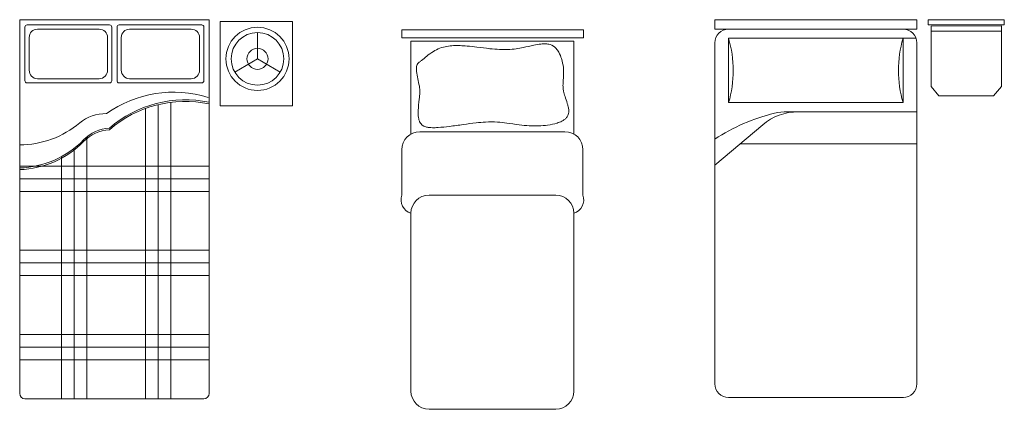
# Model space of a CAD drawing. Units: inches. Extents: x 1994 to 3075, y 3517 to 3950.
# Tile 11 of 58: x 1994.3296 to 1994.5407, y 3553.2315 to 3553.315. Entities that reach past the tile are written whole.
import ezdxf

# ---------------------------------------------------------------- set-up
doc = ezdxf.new("R2010")
doc.units = ezdxf.units.IN
doc.layers.add('A-FURN-REFR', color=8, linetype='Continuous', lineweight=13)

msp = doc.modelspace()

# ---------------------------------------------------------------- linework, layer by layer
at = {"layer": 'A-FURN-REFR'}
for p, q in [((1994.370185678926, 3553.314964244441), (1994.329576990967, 3553.314964244441)), ((1994.329576990967, 3553.314964244441), (1994.329576990967, 3553.234874887633)), ((1994.348866117747, 3553.313836225331), (1994.331156217721, 3553.313836225331)), ((1994.368606452172, 3553.313836225331), (1994.350896552145, 3553.313836225331)), ((1994.370185678926, 3553.314964244441), (1994.370185678926, 3553.234874887633)), ((1994.478602848426, 3553.314914551347), (1994.521910079674, 3553.314920144558)), ((1994.478603102663, 3553.312946047427), (1994.478602848426, 3553.314914551347)), ((1994.521910188973, 3553.312950623674), (1994.521910079674, 3553.314920144558)), ((1994.52435569552, 3553.314916554879), (1994.540668217137, 3553.314918661672)), ((1994.524355834575, 3553.313839871399), (1994.52435569552, 3553.314916554879)), ((1994.524355834575, 3553.313839871399), (1994.540668356192, 3553.313841978191)), ((1994.5249825969, 3553.313615310058), (1994.540041651892, 3553.313617254961)), ((1994.540041651892, 3553.313617254961), (1994.54004332985, 3553.300625129086)), ((1994.540668356192, 3553.313841978191), (1994.540668217137, 3553.314918661671)), ((1994.330705010077, 3553.313385017688), (1994.330705010077, 3553.301879222766)), ((1994.346610079528, 3553.312933810043), (1994.333412255941, 3553.312933810043)), ((1994.349317325391, 3553.301879222766), (1994.349317325391, 3553.313385017688)), ((1994.350445344501, 3553.313385017688), (1994.350445344501, 3553.301879222766)), ((1994.366350413952, 3553.312933810043), (1994.353152590365, 3553.312933810043)), ((1994.369057659816, 3553.301879222766), (1994.369057659816, 3553.313385017688)), ((1994.38056212126, 3553.312215362403), (1994.38056212126, 3553.306575266854)), ((1994.478603102663, 3553.312946047427), (1994.521910188842, 3553.312951640618)), ((1994.5249825969, 3553.313615310058), (1994.524984274856, 3553.300623184182)), ((1994.524982738188, 3553.312521342884), (1994.540041793181, 3553.312523287789)), ((1994.331607425365, 3553.311128979467), (1994.331607425365, 3553.304135260986)), ((1994.348414910103, 3553.304135260986), (1994.348414910103, 3553.311128979467)), ((1994.351347759789, 3553.311128979467), (1994.351347759789, 3553.304135260986)), ((1994.368155244528, 3553.304135260986), (1994.368155244528, 3553.311128979467)), ((1994.448401600234, 3553.310391664947), (1994.413453017272, 3553.310391664947)), ((1994.413453017272, 3553.310391664947), (1994.413453017272, 3553.290455538603)), ((1994.448401600234, 3553.310391664947), (1994.448401600234, 3553.290455538603)), ((1994.478612611088, 3553.236961796068), (1994.478603484016, 3553.309993291545)), ((1994.521741212387, 3553.31098311484), (1994.481556112778, 3553.310977924859)), ((1994.481556112778, 3553.310977924859), (1994.48155789243, 3553.297198397415)), ((1994.518959466981, 3553.297202210954), (1994.518957687329, 3553.310981738399)), ((1994.521910570327, 3553.309997867792), (1994.521919697399, 3553.236966372316)), ((1994.375677655234, 3553.303755219079), (1994.38056212126, 3553.306575266854)), ((1994.385446587286, 3553.303755219079), (1994.38056212126, 3553.306575266854)), ((1994.331156217721, 3553.301428015121), (1994.348866117747, 3553.301428015121)), ((1994.333412255941, 3553.30233043041), (1994.346610079528, 3553.30233043041)), ((1994.350896552145, 3553.301428015121), (1994.368606452172, 3553.301428015121)), ((1994.353152590365, 3553.30233043041), (1994.366350413952, 3553.30233043041)), ((1994.524984274856, 3553.300623184182), (1994.526657757425, 3553.298654896362)), ((1994.538370355752, 3553.298656409065), (1994.54004332985, 3553.300625129086)), ((1994.359289826759, 3553.296769779996), (1994.359289826759, 3553.233746868524)), ((1994.361997072623, 3553.297259562664), (1994.361997072623, 3553.233746868524)), ((1994.48155789243, 3553.297198397415), (1994.518959170259, 3553.29720322786)), ((1994.526657757425, 3553.298654896362), (1994.538370355752, 3553.298656409065)), ((1994.356582580895, 3553.295958376947), (1994.356582580895, 3553.233746868524)), ((1994.521912476966, 3553.295235105331), (1994.49414155207, 3553.295231518664)), ((1994.446460012292, 3553.290975785524), (1994.415394605214, 3553.290975785524)), ((1994.478606866596, 3553.283802582117), (1994.488875350771, 3553.292453532399)), ((1994.343948766863, 3553.289817339641), (1994.343948766863, 3553.233746868524)), ((1994.521913366791, 3553.288345341608), (1994.484019666392, 3553.288340447566)), ((1994.341241520999, 3553.28740160715), (1994.341241520999, 3553.233746868524)), ((1994.411511429329, 3553.28709260964), (1994.411511429329, 3553.277384669928)), ((1994.450343188176, 3553.277384669928), (1994.450343188176, 3553.28709260964)), ((1994.338534275135, 3553.285640265894), (1994.338534275135, 3553.233746868524)), ((1994.370185678926, 3553.283605313184), (1994.329576990967, 3553.283605313184)), ((1994.370185678926, 3553.28089806732), (1994.329576990967, 3553.28089806732)), ((1994.370185678926, 3553.278190821456), (1994.329576990967, 3553.278190821456)), ((1994.417336193156, 3553.277384669928), (1994.444518424349, 3553.277384669928)), ((1994.413453017272, 3553.273501494043), (1994.413453017272, 3553.235376388787)), ((1994.448401600234, 3553.235376388787), (1994.448401600234, 3553.273501494043)), ((1994.370185678926, 3553.265557007425), (1994.329576990967, 3553.265557007425)), ((1994.370185678926, 3553.262849761561), (1994.329576990967, 3553.262849761561)), ((1994.370185678926, 3553.260142515696), (1994.329576990967, 3553.260142515696)), ((1994.370185678926, 3553.247508701665), (1994.329576990967, 3553.247508701665)), ((1994.370185678926, 3553.244801455801), (1994.329576990967, 3553.244801455801)), ((1994.370185678926, 3553.242094209937), (1994.329576990967, 3553.242094209937)), ((1994.369057659816, 3553.233746868524), (1994.330705010077, 3553.233746868524)), ((1994.519044811687, 3553.234014262032), (1994.481565748322, 3553.23400942154)), ((1994.417336193156, 3553.231493212902), (1994.444518424349, 3553.231493212902))]:
    msp.add_line(p, q, dxfattribs=at)
for points in [[(1994.388077714789, 3553.314567166401), (1994.372579103558, 3553.314567166401), (1994.372579103558, 3553.296485896745), (1994.388077714789, 3553.296485896745)], [(1994.411513799174, 3553.311101471077), (1994.450430347792, 3553.311101471077), (1994.450430347792, 3553.312763276653), (1994.411513799174, 3553.312763276653)]]:
    msp.add_lwpolyline(points, close=True, dxfattribs=at)
msp.add_lwpolyline([(1994.415717140901, 3553.306221031559, -0.0071144536033679), (1994.416830524292, 3553.307136923001, -0.0291750801621191), (1994.418272017925, 3553.308160858666, -0.0995108413985327), (1994.421172431712, 3553.30925043835, -0.0309960537166681), (1994.422580733602, 3553.309406082746, -0.0213742242213407), (1994.424025083548, 3553.309416868291, -0.0138154102423473), (1994.425477869293, 3553.30932585958, -0.0092840040629771), (1994.427616086483, 3553.30909097738, 0.0043536539427215), (1994.430382063773, 3553.308755920688, 0.014634740864433), (1994.43244936847, 3553.308592984115, 0.0438384142680896), (1994.436015633939, 3553.308726752635, 0.0205965805776953), (1994.437522836489, 3553.308989654272, -0.0030532405795762), (1994.43982883519, 3553.309510514755, -0.0258862363996294), (1994.441307999698, 3553.30975390412, -0.0372674858245903), (1994.442342421448, 3553.309787357306, -0.0594222537962098), (1994.443283315345, 3553.309630668138, -0.1390712479793723), (1994.444575160915, 3553.308807129298, -0.0586638411555205), (1994.445166100647, 3553.307983348355, -0.0528613955005662), (1994.445743360173, 3553.306621725756, -0.0903311740027589), (1994.446177062131, 3553.302810669614, 0.0023761187996274), (1994.446069543849, 3553.301409835136, 0.0350786422935007), (1994.446080262775, 3553.300361830441, 0.0301021961769406), (1994.446193545359, 3553.299637858405, 0.0242628626286148), (1994.446496227885, 3553.298521961266, -0.0025129695723871), (1994.446969847513, 3553.297043305117, -0.016683843633439), (1994.447160354396, 3553.296335872206, -0.031042526979895), (1994.447274765204, 3553.295666265365, -0.1077433275196103), (1994.447189851161, 3553.294622835333, -0.0971969509952781), (1994.446835994608, 3553.294004616111, -0.0572188880031632), (1994.446385582422, 3553.293587640181, -0.0413009457476749), (1994.445812123817, 3553.293234952154, -0.0430763729579249), (1994.444773120372, 3553.292816983652, -0.0420582544055731), (1994.442762307514, 3553.292380438816, -0.0495548008396401), (1994.438805955694, 3553.292239582801, -0.0176483592672042), (1994.436665275761, 3553.292444104455, -0.0018432574081804), (1994.433985367609, 3553.292815578701, 0.0158524255451982), (1994.43204139292, 3553.293019261201, 0.0296706768072246), (1994.429448007234, 3553.293025570407, 0.0142130398266808), (1994.427456086711, 3553.29286037947, 0.0071404775766546), (1994.424675961824, 3553.292507505704, -0.0039170474728025), (1994.421683320919, 3553.292110452283, -0.0124176775830428), (1994.419263257741, 3553.291861204865, -0.0214267812853995), (1994.41806435162, 3553.291824593835, -0.0259849889690267), (1994.417321753347, 3553.291875388679, -0.0396653445020058), (1994.416653118596, 3553.292009335013, -0.2391240642373063), (1994.415323131073, 3553.293094547253, -0.0526178150763782), (1994.415128082925, 3553.293693775242, -0.0348338633937756), (1994.415030081924, 3553.294379871292, -0.0316331286276026), (1994.415020000411, 3553.2955210265, -0.0170430167712775), (1994.415237932306, 3553.297918818028, 0.0194593935250652), (1994.415342939074, 3553.2993814271, 0.0425716315945425), (1994.415270391061, 3553.30073702966, -0.0315728479582929), (1994.41467866575, 3553.303884359247, -0.0408804555025011), (1994.414648081667, 3553.304650098184, -0.0594404672514954), (1994.414737112971, 3553.305180186531, -0.1725909739171879), (1994.415225176221, 3553.305856330223, 0.01273912279684), (1994.415717140901, 3553.306221031559)], format="xyb", dxfattribs=at)
for radius in [0.0067681146598248, 0.005640095549854, 0.0022560382199416]:
    msp.add_circle((1994.38056212126, 3553.306575266854), radius, dxfattribs=at)
for centre, radius, start, end in [((1994.331156217721, 3553.313385017688), 0.0004512076439886, 90, 180), ((1994.348866117747, 3553.313385017688), 0.0004512076439886, 0, 90), ((1994.350896552145, 3553.313385017688), 0.0004512076439886, 90, 180), ((1994.368606452172, 3553.313385017688), 0.0004512076439886, 0, 90), ((1994.333412255941, 3553.311128979467), 0.0018048305759536, 90, 180), ((1994.346610079528, 3553.311128979467), 0.0018048305759529, 0, 90), ((1994.353152590365, 3553.311128979467), 0.0018048305759536, 90, 180), ((1994.366350413952, 3553.311128979467), 0.0018048305759529, 0, 90), ((1994.333412255941, 3553.304135260986), 0.0018048305759529, 180, 270), ((1994.346610079528, 3553.304135260986), 0.0018048305759529, 270, 0), ((1994.353152590365, 3553.304135260986), 0.0018048305759529, 180, 270), ((1994.366350413952, 3553.304135260986), 0.0018048305759529, 270, 0), ((1994.331156217721, 3553.301879222766), 0.0004512076439886, 180, 270), ((1994.348866117747, 3553.301879222766), 0.0004512076439879, 270, 0), ((1994.350896552145, 3553.301879222766), 0.0004512076439886, 180, 270), ((1994.368606452172, 3553.301879222766), 0.0004512076439879, 270, 0), ((1994.362573607713, 3553.274580434349), 0.0248643078922148, 72.67323284139673, 125.4131583510985), ((1994.365063151315, 3553.272935583567), 0.0248643078922151, 78.11082488000187, 130.8507503895504), ((1994.365063151315, 3553.272585021769), 0.0248643078922151, 78.11082488000187, 130.8507503895504), ((1994.347915887932, 3553.286359122003), 0.0084892637790308, 88.31488457294456, 130.1474966377413), ((1994.329418589182, 3553.308425352516), 0.0203043439794747, 270.4469903483083, 309.8984118510295), ((1994.349355225248, 3553.283272279883), 0.0084892637790316, 93.75247661138384, 135.5850886757822), ((1994.349355225248, 3553.282921718084), 0.0084892637790312, 93.75247661138384, 135.5850886757822), ((1994.415394605214, 3553.28709260964), 0.0038831758847, 90, 180), ((1994.446460012292, 3553.28709260964), 0.0038831758847, 0, 90), ((1994.328850135448, 3553.30348638096), 0.0203043439794744, 272.0515143731883, 315.3360038894048), ((1994.328850135448, 3553.303135819162), 0.0203043439794744, 272.0515143731883, 315.3360038894048), ((1994.414423811242, 3553.276413875956), 0.0030699200876728, 161.565051177078, 251.565051177078), ((1994.417336193156, 3553.273501494043), 0.0038831758847, 90, 180), ((1994.444518424349, 3553.273501494043), 0.0038831758847, 0, 90), ((1994.447430806262, 3553.276413875956), 0.0030699200876728, 288.434948822922, 18.43494882292201), ((1994.330705010077, 3553.234874887633), 0.0011280191099708, 180, 270), ((1994.369057659816, 3553.234874887633), 0.0011280191099708, 270, 0), ((1994.417336193156, 3553.235376388787), 0.0038831758847, 180, 270), ((1994.444518424349, 3553.235376388787), 0.0038831758847, 270, 0)]:
    msp.add_arc(centre, radius, start, end, dxfattribs=at)
for centre, major_axis, ratio, start_param, end_param in [((1994.481556239896, 3553.309993672899), (-0.0020879137237267, -0.0020879137237267), 0.9999999999612041, 3.927119968747128, 5.497916295600241), ((1994.518957814447, 3553.309997486439), (-0.0020879137239321, -0.0020879137239321), 0.9999999997644017, 2.356323641912046, 3.927119968845528), ((1994.457934955563, 3553.304085110305), (-0.0173992810290929, -0.0173992810290929), 0.9999999999886895, 2.072529527677572, 2.640117756443983), ((1994.542580624196, 3553.304095025509), (-0.0173992810337493, -0.0173992810337493), 0.9999999999888883, -1.06906312590559, -0.5014748971522155), ((1994.500688253728, 3553.255947134522), (-0.0283219441675507, 0.0283219441675507), 0.9999999999039649, 5.731664681785821, 6.081730710524769), ((1994.496485212309, 3553.283420797631), (-0.0083516548951192, 0.0083516548951192), 0.9999999999839913, 5.497916295660136, 6.197896823596336), ((1994.494143077486, 3553.28342049514), (-0.0083516549090922, -0.0083516549090922), 0.9999999992924022, 3.927119969226966, 4.160868355362735), ((1994.481565366968, 3553.236962177422), (0.0020879137237889, 0.0020879137237889), 0.9999999999015988, 2.356323641980645, 3.92711996877693), ((1994.518966941519, 3553.236965990961), (-0.0020879137240754, 0.0020879137240754), 0.9999999996272052, 2.356323641746435, 3.92711996901114)]:
    msp.add_ellipse(centre, major_axis=major_axis, ratio=ratio, start_param=start_param, end_param=end_param, dxfattribs=at)

doc.saveas('drawing.dxf')
